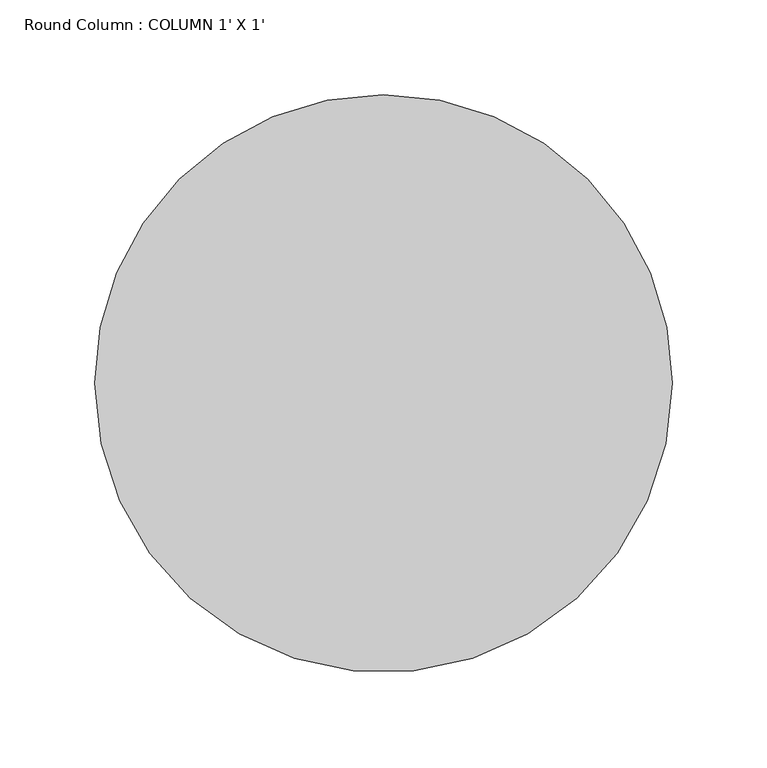
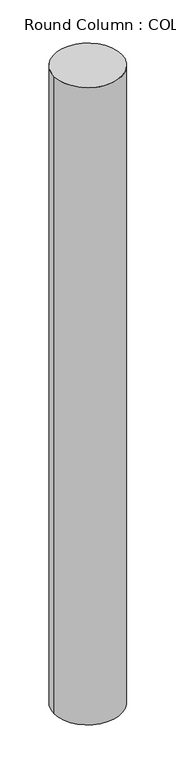
"""IFC4 building model written with IfcOpenShell, lengths in millimetres: column geometry, Round Column : COLUMN 1' X 1'."""

from ifc_helpers import new_model, si_unit, point, frame, origin, origin_2d, place, context, project, spatial, circle_curve, trimmed, segment, composite_curve, outline, extrude, source, transform, mapped, element, save


def round_column_column_1_x_1_eb224a9a(model_context):
    return source(origin(), model_context, "Body", "SweptSolid", [
        extrude(outline(composite_curve([segment(trimmed(circle_curve(origin_2d(), 152.4), [point((152.4, 0.0))], [point((-152.4, 0.0))], False, "CARTESIAN"), True, "CONTINUOUS"), segment(trimmed(circle_curve(origin_2d(), 152.4), [point((-152.4, 0.0))], [point((0.0, 152.4))], False, "CARTESIAN"), True, "CONTINUOUS"), segment(trimmed(circle_curve(origin_2d(), 152.4), [point((0.0, 152.4))], [point((152.4, 0.0))], False, "CARTESIAN"), True, "CONTINUOUS")], self_intersect=False)), frame((0.0, 0.0, 3352.8), z_axis=(0.0, 0.0, 1.0), x_axis=(1.0, 0.0, 0.0)), (0.0, 0.0, 1.0), 3048.0),
    ])


if __name__ == "__main__":
    model = new_model("IFC4")
    model_context = context("Model", 3, world=origin())
    ifc_project = project(units=[si_unit("LENGTHUNIT", "METRE", prefix="MILLI")], contexts=[model_context])
    site = spatial("IfcSite", under=ifc_project)
    building = spatial("IfcBuilding", under=site)
    placement = place(None, origin())
    round_column_column_1_x_1_shape = round_column_column_1_x_1_eb224a9a(model_context)
    element("IfcColumn", 1, ObjectType="Round Column : COLUMN 1' X 1'", at=placement, inside=building, context=model_context, shape_type="MappedRepresentation", body=[
        mapped(round_column_column_1_x_1_shape, transform((0.0, 0.0, 0.0), x_axis=(1.0, 0.0, 0.0), y_axis=(0.0, 1.0, 0.0), z_axis=(0.0, 0.0, 1.0))),
    ])
    save(model, "model.ifc")

# Revit data of these elements
# Type "Round Column : COLUMN 1' X 1'"
#   Assembly Code = "B1010200"
#   Diameter = 1' - 0"
#   Offset Base = 0' - 0"
#   Offset Top = 0' - 0"
#   Material = CREAM BEIGE COLOUR
# Element 1 (IfcColumn, "Round Column : COLUMN 1' X 1'")
#   Materials on its faces: "CREAM BEIGE COLOUR"
# Materials
#   "CREAM BEIGE COLOUR": class "Generic", colour RGB 120 120 120, transparency 0, Cost = 0
